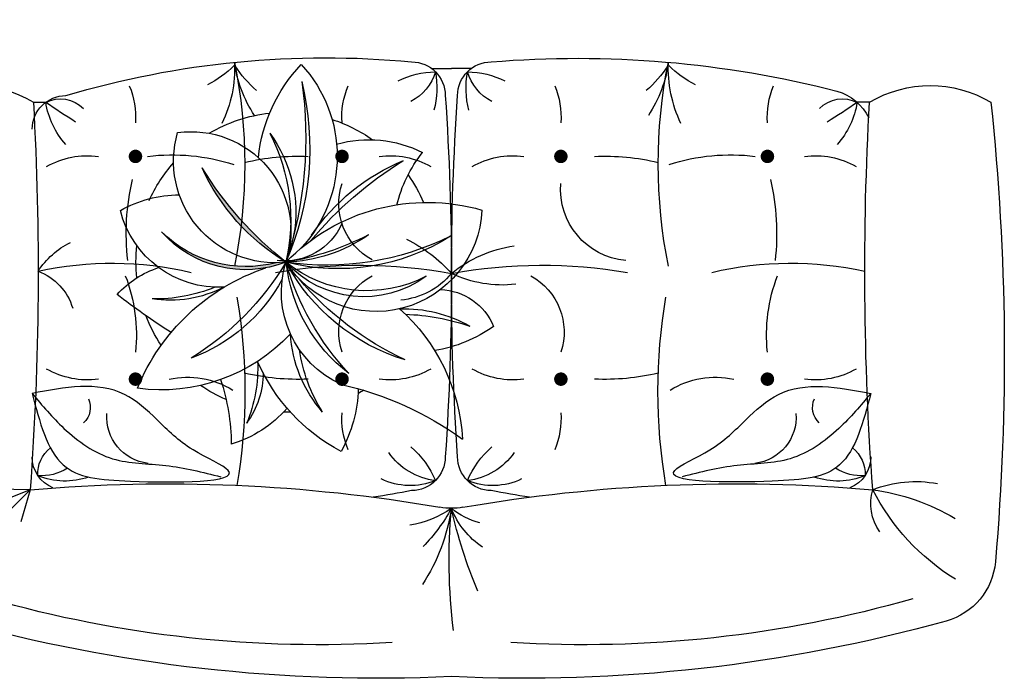
# Model space of a CAD drawing. Units: inches. Extents: x 844 to 2234, y 346 to 1084.
# Tile 50 of 93: x 1859 to 1882, y 669 to 684. Entities that reach past the tile are written whole.
import ezdxf

# ---------------------------------------------------------------- set-up
doc = ezdxf.new("R2010")
doc.units = ezdxf.units.IN
doc.header["$MEASUREMENT"] = 0
doc.layers.add('furniture', color=8, linetype='Continuous', lineweight=18)
for name, color, linetype in [('RA-AP-01$0$FURN', 3, 'Continuous'), ('RA-AP-02$0$FLPT', 30, 'Continuous'), ('ROOM-NO', 3, 'Continuous')]:
    doc.layers.add(name, color=color, linetype=linetype)

# ---------------------------------------------------------------- blocks, each defined once
blk = doc.blocks.new('A$C6E322C05')
at = {"layer": 'RA-AP-01$0$FURN'}
for p, q in [((6.391873508750865, -6.482044957760267), (6.516651486950081, -6.357266979564481)), ((6.391873508750865, -6.482044957760271), (6.43343929223883, -6.37746472106399)), ((6.391873508750866, -6.48204495776027), (6.390422568951521, -6.415535276369585)), ((6.391873508750865, -6.482044957760271), (6.439305270696451, -6.46824831830364)), ((5.817206456966433, -6.486712009544905), (5.817206456965108, -6.505053364959449)), ((5.767206456949363, -7.077520703653457), (5.767206456948565, -7.10671200954539)), ((5.767206456949363, -7.135903315437323), (5.767206456948565, -7.10671200954539)), ((5.817206456966433, -7.726712009545875), (5.817206456965108, -7.70837065413133))]:
    blk.add_line(p, q, dxfattribs=at)
at = {"layer": 'RA-AP-01$0$FURN', "const_width": 0.01}
for points in [[(5.902459393885763, -6.638129816788149, 1), (5.892459393885761, -6.638129816788122, 1)], [(6.222844373610339, -6.638129816788595, -1), (6.23284437361034, -6.638129816788595, -1)], [(5.902459393885763, -6.944444251846759, -1), (5.892459393885761, -6.944444251846785, -1)], [(6.222844373610339, -6.944444251846313, 1), (6.23284437361034, -6.944444251846313, 1)], [(5.902459393885763, -7.268979767244021, 1), (5.892459393885761, -7.268979767243994, 1)], [(6.222844373610339, -7.268979767244466, -1), (6.23284437361034, -7.268979767244466, -1)], [(5.902459393885763, -7.575294202302631, -1), (5.892459393885761, -7.575294202302657, -1)], [(6.222844373610339, -7.575294202302185, 1), (6.23284437361034, -7.575294202302185, 1)]]:
    blk.add_lwpolyline(points, format="xyb", close=True, dxfattribs=at)
at = {"layer": 'RA-AP-01$0$FURN'}
for centre, radius, start, end in [((6.192206456970573, -9.839674509409203), 3.552808610866049, 85.0473312316412, 96.0588723756579), ((5.962206456956505, -6.396712009545393), 0.1706604816468166, 148.1725534208377, 211.8274465791593), ((6.490296991311982, -6.399757455669855), 0.1, 15.49949460085664, 85.04733123164101), ((4.33669785707999, -6.99698289606033), 2.33487526667919, 357.3063521928599, 15.49949460085664), ((4.846593614069285, -6.909687157115225), 1.775196618325768, 356.4780136403396, 15.93354743557553), ((6.068281987477935, -2.019830784287151), 4.473931917517753, 266.7828902523826, 274.1477233631118), ((8.747044799885572, -6.68548500417652), 2.363941552380466, 175.0630368065897, 189.8434409139549), ((5.857266904022845, -6.534972599266733), 0.05, 90.00000000094654, 180), ((6.134026645419561, -6.595486433826224), 0.1214600988114338, 123.1053299945123, 153.7006015369794), ((6.565877894706778, -6.603111116245941), 0.5100538472773755, 167.6182489359307, 193.3122231353938), ((6.14746341585187, -6.463466129962243), 0.0853281020358404, 200.7831020638199, 253.0462459140071), ((6.367926665937501, -6.54114871013533), 0.0478550828899777, 86.575295631534, 142.6833829238214), ((6.343036863464309, -6.534972599266733), 0.05, 22.58267242460392, 89.99999999905346), ((6.302747869360707, -6.499593011892033), 0.0683206773889159, 326.6729861493449, 5.218395042636973), ((6.274768375315671, -6.53387763124781), 0.1042084262671507, 340.4828318717155, 22.86929393278168), ((5.860011614985668, -6.526983908613928), 0.0479292786975047, 152.8070868543555, 225.4025460716553), ((5.798239671935704, -6.625433523557484), 0.1218651776285568, 48.0375529564433, 81.0462320954125), ((4.904259194880517, -7.136565421857206), 1.11020813118073, 31.93286085977143, 34.66647731879807), ((6.017778833798976, -6.566879816788349), 0.1214118203512435, 150.1419074485596, 187.691663289156), ((6.107524933697323, -6.566879816788473), 0.1214118203512435, 352.3083367106845, 29.85809255128089), ((7.09459581372041, -6.919286936999045), 1.343470592134322, 163.3777289595395, 185.4806594039327), ((6.269780256940199, -6.54020363968894), 0.0310151388417235, 245.7760318513891, 317.3789451550392), ((6.284290296802319, -6.664490968717984), 0.0689028341546707, 6.419517109091462, 94.46157264568865), ((6.011601695098697, -6.976164478788355), 0.3517162425384579, 83.41248966761121, 103.1674570565571), ((6.162348040003244, -6.395238182300004), 0.2442261434243043, 248.9017070735605, 275.9923925191661), ((5.839565409091811, -6.517091257029312), 0.1212957045587361, 247.3375839744822, 273.7314750942433), ((6.197523316847625, -6.692545952238853), 0.3023568492824586, 173.0944825511667, 197.588060785551), ((6.354517986346992, -6.715077923337803), 0.1295083186917369, 167.9901339202812, 211.3796151021958), ((5.650260521516567, -6.673548227893377), 0.1579426672576338, 315.4052081938554, 333.0844958846701), ((5.765922189292775, -6.593612516654137), 0.1915923630277471, 267.5852697713958, 295.5830728418392), ((5.908792452070163, -6.03459657477793), 0.765467899454341, 258.6273206109321, 281.4174148186357), ((5.73314461686815, -6.969744817001631), 0.1863549309199891, 56.29262493376822, 82.3818003344588), ((5.679375702373212, -6.920075501166131), 0.1579426672576338, 40.38651175517922, 58.06579944599388), ((6.245858341704271, -5.977214432993086), 0.8232838708255751, 260.2449188973366, 279.7550811026635), ((6.245792934290092, -6.879444251846194), 0.3486563571350461, 166.839178360846, 182.4657575311016), ((5.879510833205829, -6.879444251846704), 0.3486563571350461, 357.5342424690579, 13.1608216393135), ((6.80739198570858, -6.9716011229856), 0.7485435294774117, 170.3094183042209, 190.3986311369044), ((5.959527339947079, -6.859074294904489), 0.0930420630931112, 293.6025128512426, 6.610683813350465), ((5.839565409091811, -7.065482811605596), 0.1212957045587361, 86.2685249057567, 112.6624160255178), ((5.967289987028921, -7.035039638983766), 0.0953802309589454, 28.80342840007747, 108.2253060204472), ((6.158013780467433, -7.035039638983501), 0.0953802309589454, 71.7746939797123, 151.196571600082), ((6.285738358404627, -7.065482811604976), 0.1212957045587361, 67.33758397464167, 93.73147509440282), ((5.08702348459791, -6.791287034316994), 1.330927509443381, 348.8964178164725, 351.3771209523497), ((6.017778833798976, -7.015694251846559), 0.1214118203512435, 172.308336710844, 209.8580925514404), ((6.107524933697323, -7.015694251846435), 0.1214118203512435, 330.1419074487191, 7.691663289315497), ((6.286338558013386, -7.045586518350251), 0.0993499474027353, 337.9047121936679, 25.63436525513283), ((6.280014948979332, -7.094901076442985), 0.0990996950214925, 6.922564260119504, 55.10883789097723), ((5.904234274973987, -7.085727051545815), 0.1323517050571434, 153.8887786398558, 178.8006589660143), ((5.999456242224805, -7.021102361717039), 0.1116589361851176, 309.9425663137084, 354.6905921774272), ((5.807266904022846, -7.047601469367252), 0.05, 180, 269.9999999990534), ((5.751472800077547, -7.013313769593298), 0.07258027258109, 286.3558526771587, 332.6774804096085), ((6.211136556040091, -6.947122539501678), 0.212288550941915, 205.9704430982785, 228.7419974602242), ((6.4323439288987, -6.955317466880212), 0.1385734111998875, 221.2288777133949, 247.0867614897648), ((6.343036863466045, -7.047601469376512), 0.05, 269.9999999989608, 359.9999999989431), ((6.304557655687245, -7.024767404076127), 0.1410608784479501, 324.4849629611242, 351.797284145529), ((6.374625390672053, -6.818147225624045), 0.2920141296149301, 278.8152064253152, 302.6921045175205), ((6.285596300104752, -6.865193601455727), 0.2760944594998999, 298.9825510110601, 313.6694461006315), ((5.795585623761384, -6.952739633017071), 0.1323517050571434, 259.6959164764198, 284.6077968025783), ((6.319376003798462, -7.10671200954539), 0.1, 350.1565590860452, 9.843440913955273), ((6.075151883811576, -3.163731520221818), 3.942980489323571, 266.1043400737264, 273.8956599242929), ((6.075151883808545, -11.04969249895812), 3.942980489412734, 86.10434007575122, 93.89565992614118), ((6.213892115887508, -7.225151532818968), 0.1854874288882049, 140.3167953258794, 172.0522897837384), ((6.80739198570858, -7.241822896105179), 0.7485435294774117, 169.6010516837189, 189.690581695779), ((5.911254573522987, -7.182496879996349), 0.1769409696162427, 353.679636560008, 25.3608296845614), ((6.496371549498975, -7.961935855380467), 0.8586827939016008, 83.03755924582121, 95.14445252709366), ((6.375720249476352, -7.220682794696101), 0.1220457486080966, 33.71356548940426, 69.04099283815023), ((6.338324584842819, -7.175279287582296), 0.1061640434993627, 14.36483859718907, 40.23030537468725), ((6.269502792941208, -7.789055933740261), 0.6986094833441214, 67.00911261779231, 77.61200156369726), ((4.336697857080025, -7.216441123030454), 2.334875266679154, 344.5005053991432, 2.69364780714023), ((5.807266904022846, -7.165822549723527), 0.05, 90.00000000094654, 180), ((6.343036863466045, -7.165822549714267), 0.05, 1.0568602e-09, 90.00000000103913), ((8.747044799885572, -7.527939014914259), 2.363941552380466, 170.156559086045, 184.9369631934102), ((5.795585623761384, -7.260684386073708), 0.1323517050571434, 75.39220319742172, 100.3040835235802), ((5.904234274973987, -7.127696967544965), 0.1323517050571434, 181.1993410339857, 206.1112213601442), ((5.751472800077547, -7.200110249497481), 0.07258027258109, 27.32251959039153, 73.64414732284132), ((6.017778833798976, -7.19772976724422), 0.1214118203512435, 150.1419074485596, 187.691663289156), ((6.107524933697323, -7.197729767244345), 0.1214118203512435, 352.3083367106845, 29.85809255128088), ((6.4323439288987, -7.25810655221026), 0.1385734111998875, 112.9132385102352, 138.7711222866051), ((6.280014948979332, -7.118522942647487), 0.0990996950214925, 304.8911621090228, 353.0774357398805), ((6.286338558013386, -7.167837500740221), 0.0993499474027353, 334.3656347448672, 22.09528780633203), ((7.290981934450236, -7.293982589837588), 1.539060359583382, 175.2233567466078, 194.4661216781742), ((5.08702348459791, -7.422136984773786), 1.330927509443381, 8.62287904765033, 11.10358218352746), ((4.846593614069285, -7.303736861975558), 1.775196618325768, 344.0664525644245, 3.521986359660393), ((6.158013780467433, -7.178384380107278), 0.0953802309589454, 208.803428399918, 288.2253060202877), ((5.839565409091811, -7.147941207485184), 0.1212957045587361, 247.3375839744822, 273.7314750942433), ((5.946346035540796, -7.374645549675604), 0.1060388135390937, 5.185910074000148, 94.80734315124221), ((6.285738358404627, -7.147941207485803), 0.1212957045587361, 266.2685249055972, 292.6624160253583), ((6.245792934290092, -7.333979767244585), 0.3486563571350461, 177.5342424688983, 193.160821639154), ((5.879510833205829, -7.333979767244075), 0.3486563571350461, 346.8391783606865, 2.465757530942165), ((5.73314461686815, -7.243679202089149), 0.1863549309199891, 277.6181996655412, 303.7073750662318), ((5.679375702373212, -7.293348517924648), 0.1579426672576338, 301.9342005540061, 319.6134882448208), ((5.908792452070163, -8.17882744431285), 0.765467899454341, 78.58258518136427, 101.3726793890678), ((6.245858341704271, -8.236209586097694), 0.8232838708255751, 80.24491889733653, 99.75508110266345), ((5.765922189292775, -7.619811502436642), 0.1915923630277471, 64.41692715816083, 92.41473022860427), ((5.650260521516567, -7.539875791197403), 0.1579426672576338, 26.91550411532996, 44.59479180614462), ((6.197523316847625, -7.520878066851927), 0.3023568492824586, 162.411939214449, 186.9055174488332), ((6.354517986346992, -7.498346095752976), 0.1295083186917369, 148.6203848978042, 192.0098660797188), ((6.565877894706778, -7.610312902844838), 0.5100538472773755, 166.6877768646062, 192.3817510640693), ((6.284290296802319, -7.548933050372795), 0.0689028341546707, 265.5384273543114, 353.5804828909086), ((5.839565409091811, -7.696332762061468), 0.1212957045587361, 86.26852490575668, 112.6624160255178), ((6.162348040003244, -7.818185836790775), 0.2442261434243043, 84.00760748083387, 111.0982929264395), ((6.011601695098697, -7.237259540302424), 0.3517162425384579, 256.8325429434429, 276.5875103323888), ((6.017778833798976, -7.646544202302431), 0.1214118203512435, 172.308336710844, 209.8580925514404), ((6.107524933697323, -7.646544202302306), 0.1214118203512435, 330.1419074487191, 7.691663289315504), ((6.269780256940199, -7.67322037940184), 0.0310151388417235, 42.62105484496073, 114.2239681486109), ((6.274768375315671, -7.679546387842969), 0.1042084262671507, 337.1307060672183, 19.51716812828453), ((5.860011614985668, -7.686440110476851), 0.0479292786975047, 134.5974539283447, 207.1929131456445), ((4.904259194880517, -7.076858597233573), 1.11020813118073, 325.333522681202, 328.0671391402286), ((5.87316911435942, -7.657653239374848), 0.0753785023123622, 196.0166452769965, 244.1254380939442), ((5.798239671935704, -7.587990495533295), 0.1218651776285568, 278.9537679045876, 311.9624470435567), ((6.302747869360707, -7.713831007198747), 0.0683206773889159, 354.781604957363, 33.32701385065516), ((6.367926665937501, -7.672275308955449), 0.0478550828899777, 217.3166170761785, 273.424704368466), ((6.343036863464309, -7.678451419824046), 0.05, 270.0000000009465, 337.4173275753961), ((6.068281987477935, -12.19359323480363), 4.473931917517753, 85.85227663688822, 93.21710974761734), ((5.966706456956126, -7.816712009545387), 0.1744999999876311, 148.9517780040469, 211.0482219959533), ((6.549562589740832, -7.794613830093475), 0.1698955038956699, 158.1487616198804, 191.122156864055), ((6.412319729336772, -7.798818772412041), 0.0704710051510922, 53.58735038429053, 106.8661365794674), ((6.713110001951175, -7.687961227420911), 0.3241573581843151, 187.6973649013944, 210.7014325157311), ((6.237117433414106, -8.032110101276656), 0.3382138395168437, 31.74362916573515, 62.76966729059727), ((6.49029699131198, -7.813666563420925), 0.1, 274.9526687683584, 344.500505399143), ((6.192206456970577, -4.373749509681577), 3.552808610866049, 263.941127624342, 274.9526687683587)]:
    blk.add_arc(centre, radius, start, end, dxfattribs=at)
for points, knots in [([(6.249068123947751, -6.484897777661085), (6.239897409094627, -6.533353418276971), (6.226611264288107, -6.603553906267942), (6.290696373977354, -6.673990528916563), (6.332121563214334, -6.713363084361603), (6.381789098403072, -6.831232979612737), (6.381738454094183, -6.629656072516828), (6.370771929626907, -6.516634365426866), (6.291185937762818, -6.495880800642047), (6.249068123947751, -6.484897777661087)], [0, 0, 0, 0, 0.1367586589314792, 0.1981301758052368, 0.2677729570689282, 0.3281194902553322, 0.4737578340741565, 0.5765194025309516, 0.6920332287422236, 0.6920332287422236, 0.6920332287422236, 0.6920332287422236]), ([(6.249068123947751, -6.484897777661087), (6.266851662635476, -6.499857019491296), (6.306238891621481, -6.532988956490432), (6.353826300430336, -6.600137645661404), (6.352465874908733, -6.685122080531377), (6.365878290565239, -6.737689715716581), (6.372748706337224, -6.764617117843226)], [0, 0, 0, 0, 0.070018540671015, 0.1550780383534498, 0.2344491945777043, 0.3178048737568289, 0.3178048737568289, 0.3178048737568289, 0.3178048737568289]), ([(6.249068123947751, -7.728526241429694), (6.239897409094627, -7.680070600813808), (6.226611264288107, -7.609870112822835), (6.290696373977354, -7.539433490174218), (6.332121563214334, -7.500060934729178), (6.381789098403072, -7.382191039478041), (6.381738454094183, -7.583767946573952), (6.370771929626907, -7.696789653663914), (6.291185937762818, -7.717543218448732), (6.249068123947751, -7.728526241429692)], [0, 0, 0, 0, 0.1367586589314792, 0.1981301758052368, 0.2677729570689282, 0.3281194902553322, 0.4737578340741565, 0.5765194025309516, 0.6920332287422236, 0.6920332287422236, 0.6920332287422236, 0.6920332287422236]), ([(6.249068123947751, -7.728526241429692), (6.266851662635476, -7.713566999599485), (6.306238891621481, -7.680435062600349), (6.353826300430336, -7.613286373429378), (6.352465874908733, -7.528301938559401), (6.365878290565239, -7.475734303374198), (6.372748706337224, -7.448806901247554)], [0, 0, 0, 0, 0.070018540671015, 0.1550780383534498, 0.2344491945777043, 0.3178048737568289, 0.3178048737568289, 0.3178048737568289, 0.3178048737568289])]:
    blk.add_open_spline(points, degree=3, knots=knots, dxfattribs=at)
blk = doc.blocks.new('A$C78016F37')
at = {"layer": 'RA-AP-02$0$FLPT'}
for points in [[(8.585816203069419, -6.02390819987247, -0.263770389754008), (8.460672408962632, -5.900531828839305, -0.0241291823863587), (8.454072418949808, -5.887595694471202, 2.53684562776e-05), (8.45404743172537, -5.887630207283394, 0.3135010205465867)], [(8.6375288720004, -5.923949758415821, -0.0887687358956854), (8.454121692088984, -5.887527659105068, 7.7903089823e-06), (8.45411401635844, -5.887538255716633, 0.1521261679004899)]]:
    blk.add_hatch(color=256, dxfattribs=at).paths.add_polyline_path(points)
at = {"layer": 'RA-AP-01$0$FURN'}
for centre, radius, start, end in [((8.676215054199671, -5.667660989702041), 0.3125591380039201, 178.1117989109854, 224.6938723266582), ((8.77416640415315, -5.62926868308301), 0.4113013577889528, 183.916601998098, 218.889069239545), ((8.454024671827373, -5.887489670112504), 0.2224048992971994, 84.85146405771819, 96.8968759960221), ((7.926806489084671, -5.648344237112944), 0.5693232143741963, 340.3683676450975, 358.6332230039188), ((8.195746570571197, -5.703566525505195), 0.3030929277970076, 334.410018118324, 8.056842366720524), ((8.454024671827373, -5.887489670112504), 0.2224048992971994, 48.29632106119188, 65.66234443375417), ((8.028579057188336, -5.942548842808446), 0.3176725093823991, 32.12276904396682, 49.65676958807643), ((8.138392155386812, -5.868774225710474), 0.1937166188785145, 28.24647600965292, 60.3482035660113), ((8.485489110864293, -5.735116799889917), 0.1555876039528135, 173.9896977683083, 258.3326220930856), ((8.521327457039675, -5.708924385009453), 0.1908277389198635, 182.9741757068071, 249.3481441545862), ((8.654249619708994, -5.778555799161595), 0.2279399438329033, 175.7401143551485, 208.5487298435666), ((8.841321835932057, -5.738299260526738), 0.4150383977849519, 183.2217031044116, 201.067141094303), ((8.454024671827373, -5.887489670112504), 0.2224048992971994, 359.5998786150253, 24.14255533511359), ((8.442163868805496, -5.589503946884691), 0.2981456377964393, 227.2393731923049, 272.0875214538299), ((8.499731284894388, -5.433816546692462), 0.4559697329776795, 235.2365058162176, 260.2774785796924), ((8.610008543493892, -6.006599373458567), 0.1961871509349957, 83.84242350983102, 130.6121505715144), ((8.645911592327788, -6.090477518425219), 0.27932894017942, 93.04938662579335, 133.3896949469156), ((8.564547574985227, -5.985184712735347), 0.1475114689626245, 22.41040215178937, 138.5254141817128), ((8.454024671827373, -5.887489670112504), 0.2224048992971994, 179.1222698891959, 181.6416201752811), ((8.343226438185093, -5.786283478281637), 0.1500631261941314, 234.481997856841, 317.590554229248), ((8.35533458686642, -5.671200371653297), 0.2372928460263133, 247.4602721701189, 294.3106346998744), ((8.353310301606033, -5.50080131865886), 0.3995888706145134, 257.1400840392136, 284.5985568218482), ((8.820839898988444, -6.089372712149781), 0.4186128907603021, 151.1845644972185, 178.7925181665867), ((8.647592804319403, -5.39327801538501), 0.5307671632505924, 248.6111860886518, 268.9135435570199), ((8.591324349397098, -5.825721750746069), 0.1505539017216363, 204.2218678925879, 316.713948440902), ((8.60427433017431, -5.61130057980146), 0.3144127437625546, 241.4533621372112, 276.0713675084609), ((8.617925276426345, -5.861018191689067), 0.1660245384207697, 189.1745772070899, 258.8487542743241), ((8.650970463531563, -6.036034461900849), 0.252604074752176, 148.7548044074418, 190.1503402437527), ((8.632043935228618, -5.851861780578565), 0.1781487401371014, 195.8547118906642, 254.9602254039967), ((8.27103219642381, -5.762377687346963), 0.1942058542978326, 259.1738264472347, 296.9361074578899), ((8.242487148295718, -5.713440208635033), 0.2398180026482373, 268.1044384936476, 291.9165885710061), ((8.454024671827373, -5.887489670112504), 0.2224048992971994, 324.5751954876287, 341.8360454133948), ((8.643418645519843, -5.97565241718072), 0.1753165964770544, 183.2000241261284, 219.1319783506275), ((8.454024671827373, -5.887489670112504), 0.2224048992971994, 208.6999597596628, 211.2898901048327), ((8.447576280134497, -6.186493140077375), 0.2128537218708566, 117.7922244992203, 143.1680179163233), ((8.391080266506174, -6.106601067273632), 0.1233275614230441, 120.0065551025349, 157.0200898875673), ((8.702436309821351, -5.965526387054176), 0.2293777808440535, 187.970132899875, 211.770006950379), ((8.454024671827373, -5.887489670112504), 0.2224048992971994, 233.8814212202215, 245.0364073377333), ((8.454024671827373, -5.887489670112504), 0.2224048992971994, 294.3332330132876, 306.7022905924929), ((8.454024671827373, -5.887489670112504), 0.2224048992971994, 266.6746775461067, 279.4836973606225)]:
    blk.add_arc(centre, radius, start, end, dxfattribs=at)
at = {"layer": 'RA-AP-02$0$FLPT'}
blk.add_lwpolyline([(8.373681407360612, -5.597603282219753, 0.7334826821515817), (8.454024671827373, -5.887489670112506, 0.2766279680881699), (8.373681407360612, -5.597603282219752, 1.3559471233864)], format="xyb", dxfattribs=at)
for centre, radius, start, end in [((8.307234168263015, -5.560224752275053), 0.1974581866646199, 313.6950443365965, 339.1517930721081), ((8.39717548070647, -5.778250590985688), 0.1754354389711152, 14.56900959352841, 57.37320031926483), ((8.423880035729836, -5.687934118592295), 0.2086915776254087, 175.0742803806306, 201.2122531761669), ((8.228139151249446, -5.75774524127399), 0.0885717136803359, 32.28640253436571, 97.90409188948885), ((8.433135668112254, -6.051756800567661), 0.1760533926534347, 161.4400574260173, 193.8427700955681), ((8.41746442128814, -6.364284642428606), 0.3118134108627832, 101.9980156162763, 119.8647524560376), ((8.395985399479063, -6.084837299933293), 0.1497734353479364, 343.3485825573843, 11.74756506179821), ((8.942045887600607, -5.120169675385827), 1.085029101271162, 243.0359441902965, 248.2214525024466)]:
    blk.add_arc(centre, radius, start, end, dxfattribs=at)
at = {"layer": 'ROOM-NO'}
for centre, radius, start, end in [((8.65235909715731, -5.915275987506324), 0.2002713751519826, 77.61332513631854, 163.1649854687259), ((8.46944987509335, -5.65497750757116), 0.2349499976215632, 306.2836330402241, 344.0182681768919), ((8.897731643814414, -6.279909663508004), 0.5923422390868573, 112.2662452820337, 138.5100534847894), ((8.794175340646271, -6.133856003178959), 0.4198977696908007, 106.7322927724504, 144.0984247900076), ((8.22288024947718, -6.040653787747125), 0.2772850355038946, 71.89678357893693, 117.3860017964977), ((7.898132843717886, -6.242790504972724), 0.48979813475044, 43.05187184217114, 66.25811984072557), ((8.347851773195234, -6.064576052783105), 0.2064758371609359, 122.2147792747386, 149.2270256684313), ((8.154124515379644, -5.981454547332234), 0.314276155615234, 322.6594768637323, 11.71644421186061), ((8.609526443069848, -6.010438452646774), 0.261483616160276, 163.3494523104177, 218.1824089018609), ((8.3154997513214, -5.724318991124441), 0.2758350084868725, 238.2734303421065, 276.8355613505966), ((8.602078464955955, -5.915823919619132), 0.1507406891149966, 207.5045866236536, 286.2267783265413), ((8.468611314717652, -6.062483436674201), 0.1756006505860901, 0.6277371554985871, 30.43990742705027)]:
    blk.add_arc(centre, radius, start, end, dxfattribs=at)
blk = doc.blocks.new('A$C5D2F253E')
at = {"layer": 'RA-AP-01$0$FURN', "xscale": -1}
blk.add_blockref('A$C6E322C05', (4.620200485489021, 7.961130550668883), dxfattribs=at)
at = {"layer": 'RA-AP-02$0$FLPT', "xscale": -1, "rotation": 210.3787734063952}
blk.add_blockref('A$C78016F37', (-5.749960471669055, -8.254610923396115), dxfattribs=at)

msp = doc.modelspace()

# ---------------------------------------------------------------- block references
at = {"layer": 'furniture', "xscale": 15.94108302203742, "yscale": 15.94108302203742, "zscale": 15.94108302203742, "rotation": 90}
msp.add_blockref('A$C5D2F253E', (1882.631064852549, 701.4028671565849), dxfattribs=at)

doc.saveas('drawing.dxf')
